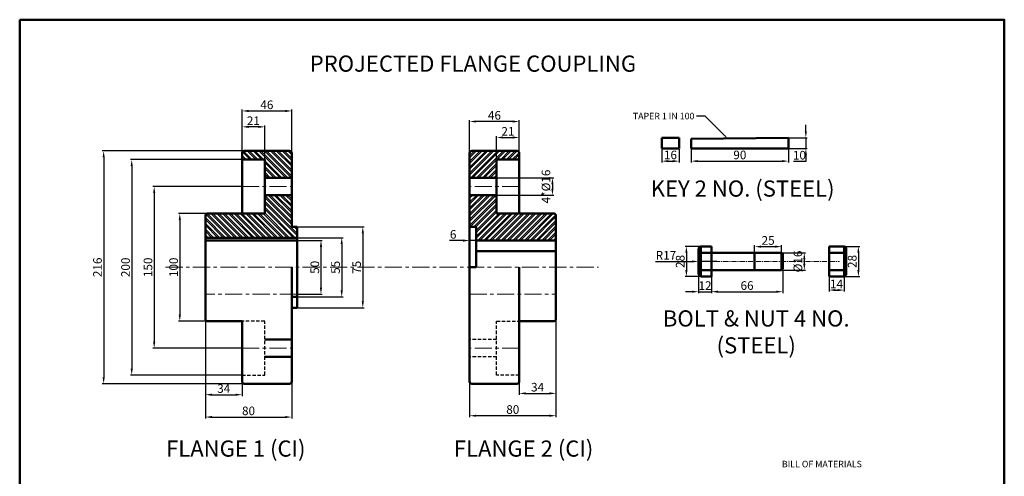
# Model space of a CAD drawing. Units: millimetres. Extents: x 36 to 952, y -590 to 448.
# Tile 2 of 2: x 39 to 952, y 24 to 448. Entities that reach past the tile are written whole.
import ezdxf
from ezdxf import colors
from ezdxf.entities.mleader import LeaderData, LeaderLine
from ezdxf.math import Vec2, Vec3

# ---------------------------------------------------------------- set-up
doc = ezdxf.new("R2010")
doc.units = ezdxf.units.MM
doc.header["$LTSCALE"] = 0.5
doc.linetypes.add('CENTER', pattern=[50.8, 31.75, -6.35, 6.35, -6.35])
doc.linetypes.add('HIDDEN', pattern=[9.525, 6.35, -3.175])
for name, color, linetype, lineweight in [('M-CNTR', 1, 'CENTER', 18), ('M-DIMS', 2, 'Continuous', 25), ('M-HATC', 8, 'Continuous', 18), ('M-HIDN', 4, 'HIDDEN', 25), ('M-OUTL', 7, 'Continuous', 50), ('M-TEXT', 7, 'Continuous', 25)]:
    doc.layers.add(name, color=color, linetype=linetype, lineweight=lineweight)
doc.styles.get("Standard").update_dxf_attribs({"font": 'arial.ttf'})
doc.dimstyles.new('ISO-25', dxfattribs={"dimtxt": 8, "dimasz": 6, "dimexe": 1.25, "dimexo": 0.625, "dimtad": 1, "dimtoh": 1, "dimtxsty": 'Standard', "dimcen": 2.5, "dimadec": 0, "dimazin": 0, "dimtfac": 1, "dimtmove": 0, "dimatfit": 3, "dimfxl": 1, "dimarcsym": 0})

# ---------------------------------------------------------------- blocks, each defined once
blk = doc.blocks.new('*D1')
at = {"layer": 'Defpoints', "color": 0, "ltscale": 0.3, "transparency": 16777216}
for p in [(291.54, 363.31), (245.54, 319.9), (291.54, 319.9)]:
    blk.add_point(p, dxfattribs=at)
at = {"layer": 'M-DIMS', "color": 0, "lineweight": -2, "ltscale": 0.3, "transparency": 16777216}
for p, q in [((245.54, 320.53), (245.54, 364.56)), ((251.54, 363.31), (285.54, 363.31)), ((291.54, 320.53), (291.54, 364.56))]:
    blk.add_line(p, q, dxfattribs=at)
at = {"layer": 'M-DIMS', "color": 0, "ltscale": 0.3, "transparency": 16777216}
for points in [[(251.54, 364.31), (251.54, 362.31), (245.54, 363.31)], [(285.54, 364.31), (285.54, 362.31), (291.54, 363.31)]]:
    blk.add_solid(points, dxfattribs=at)
at = {"layer": 'M-DIMS', "color": 0, "ltscale": 0.3, "transparency": 16777216, "insert": (268.54, 368.02), "char_height": 8, "attachment_point": 5}
blk.add_mtext('46', dxfattribs=at)
blk = doc.blocks.new('*D2')
at = {"layer": 'Defpoints', "color": 0, "ltscale": 0.3, "transparency": 16777216}
for p in [(245.54, 348.56), (245.54, 310.99), (266.54, 310.99)]:
    blk.add_point(p, dxfattribs=at)
at = {"layer": 'M-DIMS', "color": 0, "lineweight": -2, "ltscale": 0.3, "transparency": 16777216}
for p, q in [((245.54, 311.61), (245.54, 349.81)), ((260.54, 348.56), (251.54, 348.56)), ((266.54, 311.61), (266.54, 349.81))]:
    blk.add_line(p, q, dxfattribs=at)
at = {"layer": 'M-DIMS', "color": 0, "ltscale": 0.3, "transparency": 16777216}
for points in [[(251.54, 349.56), (251.54, 347.56), (245.54, 348.56)], [(260.54, 349.56), (260.54, 347.56), (266.54, 348.56)]]:
    blk.add_solid(points, dxfattribs=at)
at = {"layer": 'M-DIMS', "color": 0, "ltscale": 0.3, "transparency": 16777216, "insert": (256.04, 353.2), "char_height": 8, "attachment_point": 5}
blk.add_mtext('21', dxfattribs=at)
blk = doc.blocks.new('*D3')
at = {"layer": 'Defpoints', "color": 0, "ltscale": 0.3, "transparency": 16777216}
for p in [(221.05, 268.21), (187.84, 168.21), (221.05, 168.21)]:
    blk.add_point(p, dxfattribs=at)
at = {"layer": 'M-DIMS', "color": 0, "lineweight": -2, "ltscale": 0.3, "transparency": 16777216}
for p, q in [((220.43, 268.21), (186.59, 268.21)), ((187.84, 262.21), (187.84, 174.21)), ((220.43, 168.21), (186.59, 168.21))]:
    blk.add_line(p, q, dxfattribs=at)
at = {"layer": 'M-DIMS', "color": 0, "ltscale": 0.3, "transparency": 16777216}
for points in [[(186.84, 262.21), (188.84, 262.21), (187.84, 268.21)], [(186.84, 174.21), (188.84, 174.21), (187.84, 168.21)]]:
    blk.add_solid(points, dxfattribs=at)
at = {"layer": 'M-DIMS', "color": 0, "ltscale": 0.3, "transparency": 16777216, "insert": (183.13, 218.21), "char_height": 8, "attachment_point": 5, "rotation": 90}
blk.add_mtext('100', dxfattribs=at)
blk = doc.blocks.new('*D4')
at = {"layer": 'Defpoints', "color": 0, "ltscale": 0.3, "transparency": 16777216}
for p in [(245.54, 293.21), (164.09, 143.21), (245.54, 143.21)]:
    blk.add_point(p, dxfattribs=at)
at = {"layer": 'M-DIMS', "color": 0, "lineweight": -2, "ltscale": 0.3, "transparency": 16777216}
for p, q in [((244.92, 293.21), (162.84, 293.21)), ((164.09, 287.21), (164.09, 149.21)), ((244.92, 143.21), (162.84, 143.21))]:
    blk.add_line(p, q, dxfattribs=at)
at = {"layer": 'M-DIMS', "color": 0, "ltscale": 0.3, "transparency": 16777216}
for points in [[(163.09, 287.21), (165.09, 287.21), (164.09, 293.21)], [(163.09, 149.21), (165.09, 149.21), (164.09, 143.21)]]:
    blk.add_solid(points, dxfattribs=at)
at = {"layer": 'M-DIMS', "color": 0, "ltscale": 0.3, "transparency": 16777216, "insert": (159.38, 218.21), "char_height": 8, "attachment_point": 5, "rotation": 90}
blk.add_mtext('150', dxfattribs=at)
blk = doc.blocks.new('*D5')
at = {"layer": 'Defpoints', "color": 0, "ltscale": 0.3, "transparency": 16777216}
for p in [(245.54, 318.21), (143.27, 118.21), (245.54, 118.21)]:
    blk.add_point(p, dxfattribs=at)
at = {"layer": 'M-DIMS', "color": 0, "lineweight": -2, "ltscale": 0.3, "transparency": 16777216}
for p, q in [((244.92, 318.21), (142.02, 318.21)), ((143.27, 312.21), (143.27, 124.21)), ((244.92, 118.21), (142.02, 118.21))]:
    blk.add_line(p, q, dxfattribs=at)
at = {"layer": 'M-DIMS', "color": 0, "ltscale": 0.3, "transparency": 16777216}
for points in [[(142.27, 312.21), (144.27, 312.21), (143.27, 318.21)], [(142.27, 124.21), (144.27, 124.21), (143.27, 118.21)]]:
    blk.add_solid(points, dxfattribs=at)
at = {"layer": 'M-DIMS', "color": 0, "ltscale": 0.3, "transparency": 16777216, "insert": (138.56, 218.21), "char_height": 8, "attachment_point": 5, "rotation": 90}
blk.add_mtext('200', dxfattribs=at)
blk = doc.blocks.new('*D6')
at = {"layer": 'Defpoints', "color": 0, "ltscale": 0.3, "transparency": 16777216}
for p in [(268.54, 326.21), (117.28, 110.21), (268.54, 110.21)]:
    blk.add_point(p, dxfattribs=at)
at = {"layer": 'M-DIMS', "color": 0, "lineweight": -2, "ltscale": 0.3, "transparency": 16777216}
for p, q in [((267.92, 326.21), (116.03, 326.21)), ((117.28, 320.21), (117.28, 116.21)), ((267.92, 110.21), (116.03, 110.21))]:
    blk.add_line(p, q, dxfattribs=at)
at = {"layer": 'M-DIMS', "color": 0, "ltscale": 0.3, "transparency": 16777216}
for points in [[(116.28, 320.21), (118.28, 320.21), (117.28, 326.21)], [(116.28, 116.21), (118.28, 116.21), (117.28, 110.21)]]:
    blk.add_solid(points, dxfattribs=at)
at = {"layer": 'M-DIMS', "color": 0, "ltscale": 0.3, "transparency": 16777216, "insert": (112.57, 218.21), "char_height": 8, "attachment_point": 5, "rotation": 90}
blk.add_mtext('216', dxfattribs=at)
blk = doc.blocks.new('*D7')
at = {"layer": 'Defpoints', "color": 0, "ltscale": 0.3, "transparency": 16777216}
for p in [(296.54, 243.21), (296.54, 193.21), (318.69, 193.21)]:
    blk.add_point(p, dxfattribs=at)
at = {"layer": 'M-DIMS', "color": 0, "lineweight": -2, "ltscale": 0.3, "transparency": 16777216}
for p, q in [((297.17, 243.21), (319.94, 243.21)), ((318.69, 237.21), (318.69, 199.21)), ((297.17, 193.21), (319.94, 193.21))]:
    blk.add_line(p, q, dxfattribs=at)
at = {"layer": 'M-DIMS', "color": 0, "ltscale": 0.3, "transparency": 16777216}
for points in [[(317.69, 237.21), (319.69, 237.21), (318.69, 243.21)], [(317.69, 199.21), (319.69, 199.21), (318.69, 193.21)]]:
    blk.add_solid(points, dxfattribs=at)
at = {"layer": 'M-DIMS', "color": 0, "ltscale": 0.3, "transparency": 16777216, "insert": (313.98, 218.21), "char_height": 8, "attachment_point": 5, "rotation": 90}
blk.add_mtext('50', dxfattribs=at)
blk = doc.blocks.new('*D8')
at = {"layer": 'Defpoints', "color": 0, "ltscale": 0.3, "transparency": 16777216}
for p in [(296.54, 245.71), (296.54, 190.71), (337.91, 190.71)]:
    blk.add_point(p, dxfattribs=at)
at = {"layer": 'M-DIMS', "color": 0, "lineweight": -2, "ltscale": 0.3, "transparency": 16777216}
for p, q in [((297.17, 245.71), (339.16, 245.71)), ((337.91, 239.71), (337.91, 196.71)), ((297.17, 190.71), (339.16, 190.71))]:
    blk.add_line(p, q, dxfattribs=at)
at = {"layer": 'M-DIMS', "color": 0, "ltscale": 0.3, "transparency": 16777216}
for points in [[(336.91, 239.71), (338.91, 239.71), (337.91, 245.71)], [(336.91, 196.71), (338.91, 196.71), (337.91, 190.71)]]:
    blk.add_solid(points, dxfattribs=at)
at = {"layer": 'M-DIMS', "color": 0, "ltscale": 0.3, "transparency": 16777216, "insert": (333.22, 218.21), "char_height": 8, "attachment_point": 5, "rotation": 90}
blk.add_mtext('55', dxfattribs=at)
blk = doc.blocks.new('*D9')
at = {"layer": 'Defpoints', "color": 0, "ltscale": 0.3, "transparency": 16777216}
for p in [(296.54, 255.71), (296.54, 180.71), (357.45, 180.71)]:
    blk.add_point(p, dxfattribs=at)
at = {"layer": 'M-DIMS', "color": 0, "lineweight": -2, "ltscale": 0.3, "transparency": 16777216}
for p, q in [((297.17, 255.71), (358.7, 255.71)), ((357.45, 249.71), (357.45, 186.71)), ((297.17, 180.71), (358.7, 180.71))]:
    blk.add_line(p, q, dxfattribs=at)
at = {"layer": 'M-DIMS', "color": 0, "ltscale": 0.3, "transparency": 16777216}
for points in [[(356.45, 249.71), (358.45, 249.71), (357.45, 255.71)], [(356.45, 186.71), (358.45, 186.71), (357.45, 180.71)]]:
    blk.add_solid(points, dxfattribs=at)
at = {"layer": 'M-DIMS', "color": 0, "ltscale": 0.3, "transparency": 16777216, "insert": (352.75, 218.21), "char_height": 8, "attachment_point": 5, "rotation": 90}
blk.add_mtext('75', dxfattribs=at)
blk = doc.blocks.new('*D10')
at = {"layer": 'Defpoints', "color": 0, "ltscale": 0.3, "transparency": 16777216}
for p in [(456.46, 353.52), (456.46, 307.61), (502.46, 307.61)]:
    blk.add_point(p, dxfattribs=at)
at = {"layer": 'M-DIMS', "color": 0, "lineweight": -2, "ltscale": 0.3, "transparency": 16777216}
for p, q in [((456.46, 308.24), (456.46, 354.77)), ((496.46, 353.52), (462.46, 353.52)), ((502.46, 308.24), (502.46, 354.77))]:
    blk.add_line(p, q, dxfattribs=at)
at = {"layer": 'M-DIMS', "color": 0, "ltscale": 0.3, "transparency": 16777216}
for points in [[(462.46, 354.52), (462.46, 352.52), (456.46, 353.52)], [(496.46, 354.52), (496.46, 352.52), (502.46, 353.52)]]:
    blk.add_solid(points, dxfattribs=at)
at = {"layer": 'M-DIMS', "color": 0, "ltscale": 0.3, "transparency": 16777216, "insert": (479.46, 358.23), "char_height": 8, "attachment_point": 5}
blk.add_mtext('46', dxfattribs=at)
blk = doc.blocks.new('*D11')
at = {"layer": 'Defpoints', "color": 0, "ltscale": 0.3, "transparency": 16777216}
for p in [(502.46, 338.68), (481.46, 318.21), (502.46, 318.21)]:
    blk.add_point(p, dxfattribs=at)
at = {"layer": 'M-DIMS', "color": 0, "lineweight": -2, "ltscale": 0.3, "transparency": 16777216}
for p, q in [((481.46, 318.83), (481.46, 339.93)), ((487.46, 338.68), (496.46, 338.68)), ((502.46, 318.83), (502.46, 339.93))]:
    blk.add_line(p, q, dxfattribs=at)
at = {"layer": 'M-DIMS', "color": 0, "ltscale": 0.3, "transparency": 16777216}
for points in [[(487.46, 339.68), (487.46, 337.68), (481.46, 338.68)], [(496.46, 339.68), (496.46, 337.68), (502.46, 338.68)]]:
    blk.add_solid(points, dxfattribs=at)
at = {"layer": 'M-DIMS', "color": 0, "ltscale": 0.3, "transparency": 16777216, "insert": (491.96, 343.32), "char_height": 8, "attachment_point": 5}
blk.add_mtext('21', dxfattribs=at)
blk = doc.blocks.new('*D12')
at = {"layer": 'Defpoints', "color": 0, "ltscale": 0.3, "transparency": 16777216}
for p in [(456.46, 243.21), (456.46, 243.05), (462.46, 243.21)]:
    blk.add_point(p, dxfattribs=at)
at = {"layer": 'M-DIMS', "color": 0, "lineweight": -2, "ltscale": 0.3, "transparency": 16777216}
for p, q in [((450.46, 243.05), (437.93, 243.05)), ((462.46, 243.05), (456.46, 243.05)), ((456.46, 242.58), (456.46, 241.8)), ((462.46, 242.58), (462.46, 241.8)), ((468.46, 243.05), (474.46, 243.05))]:
    blk.add_line(p, q, dxfattribs=at)
at = {"layer": 'M-DIMS', "color": 0, "ltscale": 0.3, "transparency": 16777216}
for points in [[(450.46, 244.05), (450.46, 242.05), (456.46, 243.05)], [(468.46, 244.05), (468.46, 242.05), (462.46, 243.05)]]:
    blk.add_solid(points, dxfattribs=at)
at = {"layer": 'M-DIMS', "color": 0, "ltscale": 0.3, "transparency": 16777216, "insert": (441.2, 247.76), "char_height": 8, "attachment_point": 5}
blk.add_mtext('6', dxfattribs=at)
blk = doc.blocks.new('*D13')
at = {"layer": 'Defpoints', "color": 0, "ltscale": 0.3, "transparency": 16777216}
for p in [(536.46, 179.03), (456.46, 122.84), (456.46, 80.5)]:
    blk.add_point(p, dxfattribs=at)
at = {"layer": 'M-DIMS', "color": 0, "lineweight": -2, "ltscale": 0.3, "transparency": 16777216}
for p, q in [((536.46, 178.41), (536.46, 79.25)), ((456.46, 122.21), (456.46, 79.25)), ((530.46, 80.5), (462.46, 80.5))]:
    blk.add_line(p, q, dxfattribs=at)
at = {"layer": 'M-DIMS', "color": 0, "ltscale": 0.3, "transparency": 16777216}
for points in [[(462.46, 81.5), (462.46, 79.5), (456.46, 80.5)], [(530.46, 81.5), (530.46, 79.5), (536.46, 80.5)]]:
    blk.add_solid(points, dxfattribs=at)
at = {"layer": 'M-DIMS', "color": 0, "ltscale": 0.3, "transparency": 16777216, "insert": (496.46, 85.21), "char_height": 8, "attachment_point": 5}
blk.add_mtext('80', dxfattribs=at)
blk = doc.blocks.new('*D14')
at = {"layer": 'Defpoints', "color": 0, "ltscale": 0.3, "transparency": 16777216}
for p in [(502.46, 141.28), (536.46, 127.57), (536.46, 101.23)]:
    blk.add_point(p, dxfattribs=at)
at = {"layer": 'M-DIMS', "color": 0, "lineweight": -2, "ltscale": 0.3, "transparency": 16777216}
for p, q in [((502.46, 140.66), (502.46, 99.98)), ((536.46, 126.94), (536.46, 99.98)), ((508.46, 101.23), (530.46, 101.23))]:
    blk.add_line(p, q, dxfattribs=at)
at = {"layer": 'M-DIMS', "color": 0, "ltscale": 0.3, "transparency": 16777216}
for points in [[(508.46, 102.23), (508.46, 100.23), (502.46, 101.23)], [(530.46, 102.23), (530.46, 100.23), (536.46, 101.23)]]:
    blk.add_solid(points, dxfattribs=at)
at = {"layer": 'M-DIMS', "color": 0, "ltscale": 0.3, "transparency": 16777216, "insert": (519.46, 105.95), "char_height": 8, "attachment_point": 5}
blk.add_mtext('34', dxfattribs=at)
blk = doc.blocks.new('*D15')
at = {"layer": 'Defpoints', "color": 0, "ltscale": 0.3, "transparency": 16777216}
for p in [(481.46, 301.21), (481.46, 285.21), (533.18, 285.21)]:
    blk.add_point(p, dxfattribs=at)
at = {"layer": 'M-DIMS', "color": 0, "lineweight": -2, "ltscale": 0.3, "transparency": 16777216}
for p, q in [((482.09, 301.21), (534.43, 301.21)), ((533.18, 295.21), (533.18, 291.21)), ((482.09, 285.21), (534.43, 285.21))]:
    blk.add_line(p, q, dxfattribs=at)
at = {"layer": 'M-DIMS', "color": 0, "ltscale": 0.3, "transparency": 16777216}
for points in [[(532.18, 295.21), (534.18, 295.21), (533.18, 301.21)], [(532.18, 291.21), (534.18, 291.21), (533.18, 285.21)]]:
    blk.add_solid(points, dxfattribs=at)
at = {"layer": 'M-DIMS', "color": 0, "ltscale": 0.3, "transparency": 16777216, "insert": (528.25, 293.21), "char_height": 8, "attachment_point": 5, "rotation": 90}
blk.add_mtext('4*%%C16', dxfattribs=at)
blk = doc.blocks.new('*D16')
at = {"layer": 'Defpoints', "color": 0, "ltscale": 0.3, "transparency": 16777216}
for p in [(211.54, 170.21), (291.54, 168.21), (291.54, 79.25)]:
    blk.add_point(p, dxfattribs=at)
at = {"layer": 'M-DIMS', "color": 0, "lineweight": -2, "ltscale": 0.3, "transparency": 16777216}
for p, q in [((211.54, 169.58), (211.54, 78)), ((291.54, 167.58), (291.54, 78)), ((217.54, 79.25), (285.54, 79.25))]:
    blk.add_line(p, q, dxfattribs=at)
at = {"layer": 'M-DIMS', "color": 0, "ltscale": 0.3, "transparency": 16777216}
for points in [[(217.54, 80.25), (217.54, 78.25), (211.54, 79.25)], [(285.54, 80.25), (285.54, 78.25), (291.54, 79.25)]]:
    blk.add_solid(points, dxfattribs=at)
at = {"layer": 'M-DIMS', "color": 0, "ltscale": 0.3, "transparency": 16777216, "insert": (251.54, 83.96), "char_height": 8, "attachment_point": 5}
blk.add_mtext('80', dxfattribs=at)
blk = doc.blocks.new('*D17')
at = {"layer": 'Defpoints', "color": 0, "ltscale": 0.3, "transparency": 16777216}
for p in [(245.54, 123.37), (211.54, 110.21), (245.54, 99.98)]:
    blk.add_point(p, dxfattribs=at)
at = {"layer": 'M-DIMS', "color": 0, "lineweight": -2, "ltscale": 0.3, "transparency": 16777216}
for p, q in [((245.54, 122.75), (245.54, 98.73)), ((211.54, 109.58), (211.54, 98.73)), ((217.54, 99.98), (239.54, 99.98))]:
    blk.add_line(p, q, dxfattribs=at)
at = {"layer": 'M-DIMS', "color": 0, "ltscale": 0.3, "transparency": 16777216}
for points in [[(217.54, 100.98), (217.54, 98.98), (211.54, 99.98)], [(239.54, 100.98), (239.54, 98.98), (245.54, 99.98)]]:
    blk.add_solid(points, dxfattribs=at)
at = {"layer": 'M-DIMS', "color": 0, "ltscale": 0.3, "transparency": 16777216, "insert": (228.54, 104.7), "char_height": 8, "attachment_point": 5}
blk.add_mtext('34', dxfattribs=at)
blk = doc.blocks.new('*D18')
at = {"layer": 'Defpoints', "color": 0, "ltscale": 0.3, "transparency": 16777216}
for p in [(751.91, 338.49), (751.91, 328.49), (768.09, 328.49)]:
    blk.add_point(p, dxfattribs=at)
at = {"layer": 'M-DIMS', "color": 0, "lineweight": -2, "ltscale": 0.3, "transparency": 16777216}
for p, q in [((768.09, 344.49), (768.09, 350.49)), ((752.54, 338.49), (769.34, 338.49)), ((768.09, 338.49), (768.09, 328.49)), ((752.54, 328.49), (769.34, 328.49)), ((768.09, 322.49), (768.09, 316.49)), ((768.09, 316.49), (756.79, 316.49))]:
    blk.add_line(p, q, dxfattribs=at)
at = {"layer": 'M-DIMS', "color": 0, "ltscale": 0.3, "transparency": 16777216}
for points in [[(767.09, 344.49), (769.09, 344.49), (768.09, 338.49)], [(767.09, 322.49), (769.09, 322.49), (768.09, 328.49)]]:
    blk.add_solid(points, dxfattribs=at)
at = {"layer": 'M-DIMS', "color": 0, "ltscale": 0.3, "transparency": 16777216, "insert": (762.13, 321.2), "char_height": 8, "attachment_point": 5}
blk.add_mtext('10', dxfattribs=at)
blk = doc.blocks.new('*D19')
at = {"layer": 'Defpoints', "color": 0, "ltscale": 0.3, "transparency": 16777216}
for p in [(661.91, 328.49), (751.91, 328.49), (751.91, 316.75)]:
    blk.add_point(p, dxfattribs=at)
at = {"layer": 'M-DIMS', "color": 0, "lineweight": -2, "ltscale": 0.3, "transparency": 16777216}
for p, q in [((661.91, 327.86), (661.91, 315.5)), ((751.91, 327.86), (751.91, 315.5)), ((667.91, 316.75), (745.91, 316.75))]:
    blk.add_line(p, q, dxfattribs=at)
at = {"layer": 'M-DIMS', "color": 0, "ltscale": 0.3, "transparency": 16777216}
for points in [[(667.91, 317.75), (667.91, 315.75), (661.91, 316.75)], [(745.91, 317.75), (745.91, 315.75), (751.91, 316.75)]]:
    blk.add_solid(points, dxfattribs=at)
at = {"layer": 'M-DIMS', "color": 0, "ltscale": 0.3, "transparency": 16777216, "insert": (706.91, 321.46), "char_height": 8, "attachment_point": 5}
blk.add_mtext('90', dxfattribs=at)
blk = doc.blocks.new('*D20')
at = {"layer": 'Defpoints', "color": 0, "ltscale": 0.3, "transparency": 16777216}
for p in [(634.6, 328.49), (650.6, 328.49), (650.6, 316.75)]:
    blk.add_point(p, dxfattribs=at)
at = {"layer": 'M-DIMS', "color": 0, "lineweight": -2, "ltscale": 0.3, "transparency": 16777216}
for p, q in [((634.6, 327.86), (634.6, 315.5)), ((650.6, 327.86), (650.6, 315.5)), ((640.6, 316.75), (644.6, 316.75))]:
    blk.add_line(p, q, dxfattribs=at)
at = {"layer": 'M-DIMS', "color": 0, "ltscale": 0.3, "transparency": 16777216}
for points in [[(640.6, 317.75), (640.6, 315.75), (634.6, 316.75)], [(644.6, 317.75), (644.6, 315.75), (650.6, 316.75)]]:
    blk.add_solid(points, dxfattribs=at)
at = {"layer": 'M-DIMS', "color": 0, "ltscale": 0.3, "transparency": 16777216, "insert": (642.6, 321.46), "char_height": 8, "attachment_point": 5}
blk.add_mtext('16', dxfattribs=at)
blk = doc.blocks.new('*D21')
at = {"layer": 'Defpoints', "color": 0, "ltscale": 0.3, "transparency": 16777216}
for p in [(668.62, 223.66), (680.62, 223.66), (680.62, 195.58)]:
    blk.add_point(p, dxfattribs=at)
at = {"layer": 'M-DIMS', "color": 0, "lineweight": -2, "ltscale": 0.3, "transparency": 16777216}
for p, q in [((668.62, 223.04), (668.62, 194.33)), ((680.62, 223.04), (680.62, 194.33)), ((662.62, 195.58), (656.62, 195.58)), ((668.62, 195.58), (680.62, 195.58)), ((686.62, 195.58), (692.62, 195.58))]:
    blk.add_line(p, q, dxfattribs=at)
at = {"layer": 'M-DIMS', "color": 0, "ltscale": 0.3, "transparency": 16777216}
for points in [[(662.62, 196.58), (662.62, 194.58), (668.62, 195.58)], [(686.62, 196.58), (686.62, 194.58), (680.62, 195.58)]]:
    blk.add_solid(points, dxfattribs=at)
at = {"layer": 'M-DIMS', "color": 0, "ltscale": 0.3, "transparency": 16777216, "insert": (674.62, 200.22), "char_height": 8, "attachment_point": 5}
blk.add_mtext('12', dxfattribs=at)
blk = doc.blocks.new('*D22')
at = {"layer": 'Defpoints', "color": 0, "ltscale": 0.3, "transparency": 16777216}
for p in [(680.62, 215.66), (746.62, 215.66), (746.62, 195.58)]:
    blk.add_point(p, dxfattribs=at)
at = {"layer": 'M-DIMS', "color": 0, "lineweight": -2, "ltscale": 0.3, "transparency": 16777216}
for p, q in [((680.62, 215.04), (680.62, 194.33)), ((746.62, 215.04), (746.62, 194.33)), ((686.62, 195.58), (740.62, 195.58))]:
    blk.add_line(p, q, dxfattribs=at)
at = {"layer": 'M-DIMS', "color": 0, "ltscale": 0.3, "transparency": 16777216}
for points in [[(686.62, 196.58), (686.62, 194.58), (680.62, 195.58)], [(740.62, 196.58), (740.62, 194.58), (746.62, 195.58)]]:
    blk.add_solid(points, dxfattribs=at)
at = {"layer": 'M-DIMS', "color": 0, "ltscale": 0.3, "transparency": 16777216, "insert": (713.62, 200.28), "char_height": 8, "attachment_point": 5}
blk.add_mtext('66', dxfattribs=at)
blk = doc.blocks.new('*D23')
at = {"layer": 'Defpoints', "color": 0, "ltscale": 0.3, "transparency": 16777216}
for p in [(745.62, 237.4), (720.62, 231.66), (745.62, 231.66)]:
    blk.add_point(p, dxfattribs=at)
at = {"layer": 'M-DIMS', "color": 0, "lineweight": -2, "ltscale": 0.3, "transparency": 16777216}
for p, q in [((720.62, 232.29), (720.62, 238.65)), ((726.62, 237.4), (739.62, 237.4)), ((745.62, 232.29), (745.62, 238.65))]:
    blk.add_line(p, q, dxfattribs=at)
at = {"layer": 'M-DIMS', "color": 0, "ltscale": 0.3, "transparency": 16777216}
for points in [[(726.62, 238.4), (726.62, 236.4), (720.62, 237.4)], [(739.62, 238.4), (739.62, 236.4), (745.62, 237.4)]]:
    blk.add_solid(points, dxfattribs=at)
at = {"layer": 'M-DIMS', "color": 0, "ltscale": 0.3, "transparency": 16777216, "insert": (733.12, 242.11), "char_height": 8, "attachment_point": 5}
blk.add_mtext('25', dxfattribs=at)
blk = doc.blocks.new('*D24')
at = {"layer": 'Defpoints', "color": 0, "ltscale": 0.3, "transparency": 16777216}
for p in [(745.62, 231.66), (745.62, 215.66), (766.66, 215.66)]:
    blk.add_point(p, dxfattribs=at)
at = {"layer": 'M-DIMS', "color": 0, "lineweight": -2, "ltscale": 0.3, "transparency": 16777216}
for p, q in [((746.25, 231.66), (767.91, 231.66)), ((766.66, 225.66), (766.66, 221.66)), ((746.25, 215.66), (767.91, 215.66))]:
    blk.add_line(p, q, dxfattribs=at)
at = {"layer": 'M-DIMS', "color": 0, "ltscale": 0.3, "transparency": 16777216}
for points in [[(765.66, 225.66), (767.66, 225.66), (766.66, 231.66)], [(765.66, 221.66), (767.66, 221.66), (766.66, 215.66)]]:
    blk.add_solid(points, dxfattribs=at)
at = {"layer": 'M-DIMS', "color": 0, "ltscale": 0.3, "transparency": 16777216, "insert": (761.73, 223.66), "char_height": 8, "attachment_point": 5, "rotation": 90}
blk.add_mtext('%%C16', dxfattribs=at)
blk = doc.blocks.new('*D25')
at = {"layer": 'Defpoints', "color": 0, "ltscale": 0.3, "transparency": 16777216}
for p in [(789.55, 209.66), (803.55, 209.66), (803.55, 197.1)]:
    blk.add_point(p, dxfattribs=at)
at = {"layer": 'M-DIMS', "color": 0, "lineweight": -2, "ltscale": 0.3, "transparency": 16777216}
for p, q in [((789.55, 209.04), (789.55, 195.85)), ((803.55, 209.04), (803.55, 195.85)), ((795.55, 197.1), (797.55, 197.1))]:
    blk.add_line(p, q, dxfattribs=at)
at = {"layer": 'M-DIMS', "color": 0, "ltscale": 0.3, "transparency": 16777216}
for points in [[(795.55, 198.1), (795.55, 196.1), (789.55, 197.1)], [(797.55, 198.1), (797.55, 196.1), (803.55, 197.1)]]:
    blk.add_solid(points, dxfattribs=at)
at = {"layer": 'M-DIMS', "color": 0, "ltscale": 0.3, "transparency": 16777216, "insert": (796.55, 201.74), "char_height": 8, "attachment_point": 5}
blk.add_mtext('14', dxfattribs=at)
blk = doc.blocks.new('*D28')
at = {"layer": 'Defpoints', "color": 0, "ltscale": 0.5, "transparency": 16777216}
for p in [(670.62, 237.66), (657.37, 209.66), (670.62, 209.66)]:
    blk.add_point(p, dxfattribs=at)
at = {"layer": 'M-DIMS', "color": 0, "lineweight": -2, "ltscale": 0.5, "transparency": 16777216}
for p, q in [((670, 237.66), (656.12, 237.66)), ((657.37, 231.66), (657.37, 215.66)), ((670, 209.66), (656.12, 209.66))]:
    blk.add_line(p, q, dxfattribs=at)
at = {"layer": 'M-DIMS', "color": 0, "ltscale": 0.5, "transparency": 16777216}
for points in [[(656.37, 231.66), (658.37, 231.66), (657.37, 237.66)], [(656.37, 215.66), (658.37, 215.66), (657.37, 209.66)]]:
    blk.add_solid(points, dxfattribs=at)
at = {"layer": 'M-DIMS', "color": 0, "ltscale": 0.5, "transparency": 16777216, "insert": (652.66, 223.66), "char_height": 8, "attachment_point": 5, "rotation": 90}
blk.add_mtext('28', dxfattribs=at)
blk = doc.blocks.new('*D29')
at = {"layer": 'Defpoints', "color": 0, "ltscale": 0.5, "transparency": 16777216}
for p in [(803.55, 237.66), (803.55, 209.66), (816.8, 209.66)]:
    blk.add_point(p, dxfattribs=at)
at = {"layer": 'M-DIMS', "color": 0, "lineweight": -2, "ltscale": 0.5, "transparency": 16777216}
for p, q in [((804.18, 237.66), (818.05, 237.66)), ((816.8, 231.66), (816.8, 215.66)), ((804.18, 209.66), (818.05, 209.66))]:
    blk.add_line(p, q, dxfattribs=at)
at = {"layer": 'M-DIMS', "color": 0, "ltscale": 0.5, "transparency": 16777216}
for points in [[(815.8, 231.66), (817.8, 231.66), (816.8, 237.66)], [(815.8, 215.66), (817.8, 215.66), (816.8, 209.66)]]:
    blk.add_solid(points, dxfattribs=at)
at = {"layer": 'M-DIMS', "color": 0, "ltscale": 0.5, "transparency": 16777216, "insert": (812.09, 223.66), "char_height": 8, "attachment_point": 5, "rotation": 90}
blk.add_mtext('28', dxfattribs=at)
blk = doc.blocks.new('*D32')
at = {"layer": 'Defpoints', "color": 0, "ltscale": 0.5, "transparency": 16777216}
for p in [(668.62, 223.66), (685.62, 223.66)]:
    blk.add_point(p, dxfattribs=at)
at = {"layer": 'M-DIMS', "color": 0, "lineweight": -2, "ltscale": 0.5, "transparency": 16777216}
for p, q in [((628.85, 223.66), (648.59, 223.66)), ((648.59, 223.66), (662.62, 223.66)), ((685.62, 223.66), (668.62, 223.66))]:
    blk.add_line(p, q, dxfattribs=at)
at = {"layer": 'M-DIMS', "color": 0, "ltscale": 0.5, "transparency": 16777216}
blk.add_solid([(662.62, 224.66), (662.62, 222.66), (668.62, 223.66)], dxfattribs=at)
at = {"layer": 'M-DIMS', "color": 0, "ltscale": 0.5, "transparency": 16777216, "insert": (638.41, 228.3), "char_height": 8, "attachment_point": 5}
blk.add_mtext('R17', dxfattribs=at)

msp = doc.modelspace()

# ---------------------------------------------------------------- hatches: boundary and pattern name
at = {"layer": 'M-HATC', "ltscale": 0.3}
h = msp.add_hatch(dxfattribs=at)
h.set_pattern_fill('ANSI32', color=256, scale=0.4, angle=90)
h.paths.add_polyline_path([(291.545, 324.207, 0.4142136), (289.545, 326.207), (247.545, 326.207, 0.4142136), (245.545, 324.207), (245.545, 318.207), (266.545, 318.207), (266.545, 301.207), (291.545, 301.207)])
h.paths.add_polyline_path([(291.545, 285.207), (266.545, 285.207), (266.545, 268.207), (213.545, 268.207, 0.4142136), (211.545, 266.207), (211.545, 245.707), (296.545, 245.707), (296.545, 255.707), (291.545, 255.707)])
h = msp.add_hatch(dxfattribs=at)
h.set_pattern_fill('ANSI32', color=256, scale=0.4)
h.paths.add_polyline_path([(481.461, 318.207), (502.461, 318.207), (502.461, 324.207, 0.4142136), (500.461, 326.207), (458.461, 326.207, 0.4142136), (456.461, 324.207), (456.461, 301.207), (481.461, 301.207)])
h.paths.add_polyline_path([(481.461, 285.207), (456.461, 285.207), (456.461, 255.707), (462.461, 255.707), (462.461, 243.207), (536.461, 243.207), (536.461, 266.207, 0.4142136), (534.461, 268.207), (481.461, 268.207)])

# ---------------------------------------------------------------- linework, layer by layer
at = {"layer": 'M-CNTR'}
for p, q in [((245.545, 293.207), (291.545, 293.207)), ((502.461, 293.207), (456.461, 293.207)), ((174.652, 218.207), (575.862, 218.207)), ((296.545, 193.207), (211.545, 193.207)), ((456.461, 193.207), (536.461, 193.207)), ((245.545, 143.207), (291.545, 143.207)), ((502.461, 143.207), (456.461, 143.207))]:
    msp.add_line(p, q, dxfattribs=at)
at = {"layer": 'M-CNTR', "ltscale": 0.3}
msp.add_line((668.622, 223.663), (799.251, 223.663), dxfattribs=at)
at = {"layer": 'M-HIDN'}
for p, q in [((266.545, 168.207), (245.545, 168.207)), ((266.545, 118.207), (266.545, 168.207)), ((481.461, 118.207), (481.461, 168.207)), ((481.461, 168.207), (502.461, 168.207)), ((481.461, 151.207), (456.461, 151.207)), ((481.461, 135.207), (456.461, 135.207)), ((245.545, 118.207), (266.545, 118.207)), ((502.461, 118.207), (481.461, 118.207))]:
    msp.add_line(p, q, dxfattribs=at)
at = {"layer": 'M-OUTL', "ltscale": 0.3}
for p, q in [((634.597, 338.488), (650.597, 338.488)), ((634.597, 328.488), (634.597, 338.488)), ((650.597, 338.488), (650.597, 328.488)), ((661.912, 337.488), (751.912, 338.488)), ((751.912, 338.488), (751.912, 328.488)), ((661.912, 328.488), (661.912, 337.488)), ((650.597, 328.488), (634.597, 328.488)), ((751.912, 328.488), (661.912, 328.488)), ((291.545, 255.707), (296.545, 255.707)), ((456.461, 255.707), (462.461, 255.707)), ((462.461, 255.707), (462.461, 218.207)), ((456.461, 180.707), (456.461, 243.207)), ((680.622, 237.663), (670.622, 237.663)), ((670.622, 237.663), (670.622, 209.663)), ((680.622, 231.663), (680.622, 237.663)), ((803.554, 237.663), (789.554, 237.663)), ((789.554, 237.663), (789.554, 209.663)), ((803.554, 209.663), (803.554, 237.663)), ((668.622, 234.663), (668.622, 215.663)), ((668.622, 231.663), (745.622, 231.663)), ((680.622, 215.663), (680.622, 231.663)), ((720.622, 231.663), (720.622, 215.663)), ((746.622, 230.663), (745.622, 231.663)), ((745.622, 231.663), (745.622, 215.663)), ((746.622, 230.663), (746.622, 216.663)), ((803.554, 231.663), (789.554, 231.663)), ((805.554, 212.663), (805.554, 234.663)), ((291.545, 180.707), (291.545, 218.207)), ((462.461, 218.207), (456.461, 218.207)), ((745.622, 215.663), (668.622, 215.663)), ((668.622, 215.663), (668.622, 212.663)), ((680.622, 209.663), (680.622, 215.663)), ((746.622, 216.663), (745.622, 215.663)), ((803.554, 215.663), (789.554, 215.663)), ((670.622, 209.663), (680.622, 209.663)), ((789.554, 209.663), (803.554, 209.663)), ((213.545, 168.207), (245.545, 168.207)), ((534.461, 168.207), (502.461, 168.207))]:
    msp.add_line(p, q, dxfattribs=at)
at = {"layer": 'M-OUTL'}
for p, q in [((245.545, 324.207), (245.545, 268.207)), ((247.545, 326.207), (289.545, 326.207)), ((291.545, 324.207), (291.545, 255.707)), ((456.461, 324.207), (456.461, 193.207)), ((458.461, 326.207), (500.461, 326.207)), ((502.461, 324.207), (502.461, 268.207)), ((245.545, 318.207), (266.545, 318.207)), ((266.545, 318.207), (266.545, 268.207)), ((502.461, 318.207), (481.461, 318.207)), ((481.461, 318.207), (481.461, 268.207)), ((266.545, 301.207), (291.545, 301.207)), ((481.461, 301.207), (456.461, 301.207)), ((266.545, 285.207), (291.545, 285.207)), ((481.461, 285.207), (456.461, 285.207)), ((211.545, 266.207), (211.545, 218.207)), ((266.545, 268.207), (213.545, 268.207)), ((481.461, 268.207), (534.461, 268.207)), ((536.461, 266.207), (536.461, 218.207)), ((291.545, 255.707), (296.545, 255.707)), ((296.545, 255.707), (296.545, 218.207)), ((296.545, 245.707), (211.545, 245.707)), ((296.545, 243.207), (211.545, 243.207)), ((462.461, 243.207), (536.461, 243.207)), ((462.461, 233.207), (536.461, 233.207)), ((211.545, 170.207), (211.545, 218.207)), ((296.545, 180.707), (296.545, 218.207)), ((502.461, 112.207), (502.461, 218.207)), ((536.461, 170.207), (536.461, 218.207)), ((296.545, 190.707), (291.545, 190.707)), ((291.545, 112.207), (291.545, 180.707)), ((291.545, 180.707), (296.545, 180.707)), ((456.461, 112.207), (456.461, 180.707)), ((245.545, 112.207), (245.545, 168.207)), ((266.545, 151.207), (291.545, 151.207)), ((266.545, 135.207), (291.545, 135.207)), ((247.545, 110.207), (289.545, 110.207)), ((458.461, 110.207), (500.461, 110.207))]:
    msp.add_line(p, q, dxfattribs=at)
at = {"layer": 'M-OUTL', "ltscale": 0.5}
msp.add_lwpolyline([(39.441, 448.041), (952.031, 448.041), (952.031, -589.796), (39.441, -589.796)], close=True, dxfattribs=at)
at = {"layer": 'M-OUTL'}
for centre, start, end in [((247.545, 324.207), 90, 180), ((289.545, 324.207), 0, 90), ((458.461, 324.207), 90, 180), ((500.461, 324.207), 0, 90), ((213.545, 266.207), 90, 180), ((534.461, 266.207), 0, 90), ((247.545, 112.207), 180, 270), ((289.545, 112.207), 270, 360), ((458.461, 112.207), 180, 270), ((500.461, 112.207), 270, 0)]:
    msp.add_arc(centre, 2, start, end, dxfattribs=at)
at = {"layer": 'M-OUTL', "ltscale": 0.3}
for centre, radius, start, end in [((671.872, 234.663), 3.25, 112.619865, 247.380135), ((802.304, 234.663), 3.25, 292.619865, 67.380135), ((685.622, 223.663), 17, 151.927513, 208.072487), ((788.554, 223.663), 17, 331.927513, 28.072487), ((671.872, 212.663), 3.25, 112.619865, 247.380135), ((802.304, 212.663), 3.25, 292.619865, 67.380135), ((213.545, 170.207), 2, 180, 270), ((534.461, 170.207), 2, 270, 0)]:
    msp.add_arc(centre, radius, start, end, dxfattribs=at)

# ---------------------------------------------------------------- texts
at = {"layer": 'M-TEXT', "ltscale": 0.3, "char_height": 15, "attachment_point": 1}
for s, width, insert in [('\\pxqc;PROJECTED FLANGE COUPLING', 336.57627, (291.203, 414.746)), ('\\pxqc;KEY 2 NO. (STEEL)', 198.01287, (610.508, 298.808)), ('\\pxqc;BOLT & NUT 4 NO. (STEEL)', 198.01287, (623.101, 178.286)), ('\\pxqc;FLANGE 1 (CI)', 148.39271, (165.529, 57.51)), ('\\pxqc;FLANGE 2 (CI)', 148.39271, (432.289, 57.51))]:
    msp.add_mtext_dynamic_manual_height_columns(s, width=width, gutter_width=12.5, heights=[0], dxfattribs=dict(at, insert=insert))
at = {"layer": 'M-TEXT', "ltscale": 0.5, "insert": (741.671, 38.646), "char_height": 6, "attachment_point": 1}
msp.add_mtext_dynamic_manual_height_columns('\\pxqc;BILL OF MATERIALS', width=82.56299, gutter_width=12.5, heights=[0], dxfattribs=at)

# ---------------------------------------------------------------- dimensions: what is measured, and where the dimension line sits
at = {"layer": 'M-DIMS', "ltscale": 0.3}
for base, p1, p2, picture, middle in [((291.545, 363.313), (245.545, 319.905), (291.545, 319.905), '*D1', (268.545, 368.023)), ((245.545, 348.557), (266.545, 310.985), (245.545, 310.985), '*D2', (256.045, 353.199)), ((456.461, 353.519), (502.461, 307.615), (456.461, 307.615), '*D10', (479.461, 358.229)), ((502.461, 338.679), (481.461, 318.207), (502.461, 318.207), '*D11', (491.961, 343.32)), ((650.597, 316.749), (634.597, 328.488), (650.597, 328.488), '*D20', (642.597, 321.458)), ((751.912, 316.749), (661.912, 328.488), (751.912, 328.488), '*D19', (706.912, 321.458)), ((456.461, 243.048), (462.461, 243.207), (456.461, 243.207), '*D12', (441.195, 247.758)), ((745.622, 237.397), (720.622, 231.663), (745.622, 231.663), '*D23', (733.122, 242.107)), ((680.622, 195.575), (668.622, 223.663), (680.622, 223.663), '*D21', (674.622, 200.217)), ((746.622, 195.575), (680.622, 215.663), (746.622, 215.663), '*D22', (713.622, 200.285)), ((803.554, 197.102), (789.554, 209.663), (803.554, 209.663), '*D25', (796.554, 201.743)), ((456.461, 80.497), (536.461, 179.034), (456.461, 122.839), '*D13', (496.461, 85.206)), ((291.545, 79.247), (211.545, 170.207), (291.545, 168.207), '*D16', (251.545, 83.956)), ((536.461, 101.233), (502.461, 141.284), (536.461, 127.568), '*D14', (519.461, 105.945)), ((245.545, 99.983), (211.545, 110.207), (245.545, 123.371), '*D17', (228.545, 104.695))]:
    dim = msp.add_linear_dim(base=base, p1=p1, p2=p2, dimstyle='ISO-25', override={"dimclrd": 0, "dimclre": 0, "dimclrt": 0}, dxfattribs=at)
    dim.commit()
    dim.dimension.update_dxf_attribs({"geometry": picture, "text_midpoint": middle})
for base, p1, p2, picture, middle in [((768.091, 328.488), (751.912, 338.488), (751.912, 328.488), '*D18', (762.126, 321.197)), ((117.281, 110.207), (268.545, 326.207), (268.545, 110.207), '*D6', (112.572, 218.207)), ((357.445, 180.707), (296.545, 255.707), (296.545, 180.707), '*D9', (352.752, 218.207)), ((337.913, 190.707), (296.545, 245.707), (296.545, 190.707), '*D8', (333.219, 218.207)), ((318.687, 193.207), (296.545, 243.207), (296.545, 193.207), '*D7', (313.977, 218.207))]:
    dim = msp.add_linear_dim(base=base, p1=p1, p2=p2, angle=90, dimstyle='ISO-25', override={"dimclrd": 0, "dimclre": 0, "dimclrt": 0}, dxfattribs=at)
    dim.commit()
    dim.dimension.update_dxf_attribs({"geometry": picture, "text_midpoint": middle})
for base, p1, p2, picture, middle in [((143.271, 118.207), (245.545, 318.207), (245.545, 118.207), '*D5', (143.271, 218.207)), ((164.093, 143.207), (245.545, 293.207), (245.545, 143.207), '*D4', (164.093, 218.207)), ((187.838, 168.207), (221.051, 268.207), (221.051, 168.207), '*D3', (187.838, 218.207))]:
    dim = msp.add_linear_dim(base=base, p1=p1, p2=p2, angle=90, dimstyle='ISO-25', override={"dimclrd": 0, "dimclre": 0, "dimclrt": 0}, dxfattribs=at)
    dim.commit()
    dim.dimension.update_dxf_attribs({"geometry": picture, "text_midpoint": middle, "dimtype": 160})
for base, p1, p2, text, picture, middle in [((533.185, 285.207), (481.461, 301.207), (481.461, 285.207), '4*%%C<>', '*D15', (533.185, 293.207)), ((766.658, 215.663), (745.622, 231.663), (745.622, 215.663), '%%C<>', '*D24', (766.658, 223.663))]:
    dim = msp.add_linear_dim(base=base, p1=p1, p2=p2, angle=90, text=text, dimstyle='ISO-25', override={"dimclrd": 0, "dimclre": 0, "dimclrt": 0}, dxfattribs=at)
    dim.commit()
    dim.dimension.update_dxf_attribs({"geometry": picture, "text_midpoint": middle, "dimtype": 160})
at = {"layer": 'M-DIMS', "ltscale": 0.5}
for base, p1, p2, picture, middle in [((657.372, 209.663), (670.622, 237.663), (670.622, 209.663), '*D28', (652.663, 223.663)), ((816.804, 209.663), (803.554, 237.663), (803.554, 209.663), '*D29', (812.094, 223.663))]:
    dim = msp.add_linear_dim(base=base, p1=p1, p2=p2, angle=90, dimstyle='ISO-25', override={"dimdec": 0, "dimlfac": 1, "dimrnd": 0, "dimzin": 0, "dimdsep": 46, "dimlunit": 2}, dxfattribs=at)
    dim.commit()
    dim.dimension.update_dxf_attribs({"geometry": picture, "text_midpoint": middle})
dim = msp.add_radius_dim(center=(685.622, 223.663), mpoint=(668.622, 223.663), dimstyle='ISO-25', override={"dimdec": 0, "dimlfac": 1, "dimrnd": 0, "dimzin": 0, "dimdsep": 46, "dimlunit": 2}, dxfattribs=at)
dim.commit()
dim.dimension.update_dxf_attribs({"geometry": '*D32', "text_midpoint": (638.407, 228.304)})

# ---------------------------------------------------------------- leaders
at = {"layer": 'M-TEXT', "ltscale": 0.3}
ml = msp.add_multileader_mtext('Standard', dxfattribs=at)
ml.set_content('TAPER 1 IN 100', color=256)
ml.set_leader_properties()
ml.build(insert=Vec2(0, 0))
ctx = ml.context
ctx.base_point, ctx.char_height, ctx.plane_origin = Vec3(601.461, 358.546), 6, Vec3(695.509, 337.861)
ctx.text_align_type = 2
notes = []
notes.append((ctx, [(0, (1, 1, 0), (674.824, 358.546), (-1, 0), 8, [(0, [(695.509, 337.861)], 0, [])])]))
ctx.mtext.insert, ctx.mtext.alignment, ctx.mtext.flow_direction = Vec3(664.824, 361.597), 3, 5
for ctx, leaders in notes:
    for number, flags, end, landing, length, lines in leaders:
        leader = LeaderData()
        leader.index, (leader.has_last_leader_line, leader.has_dogleg_vector, leader.attachment_direction) = number, flags
        leader.last_leader_point, leader.dogleg_vector, leader.dogleg_length = Vec3(end), Vec3(landing), length
        for number, points, colour, breaks in lines:
            line = LeaderLine()
            line.index, line.vertices, line.color, line.breaks = number, Vec3.list(points), colors.encode_raw_color(colour), breaks
            leader.lines.append(line)
        ctx.leaders.append(leader)

doc.saveas('drawing.dxf')
